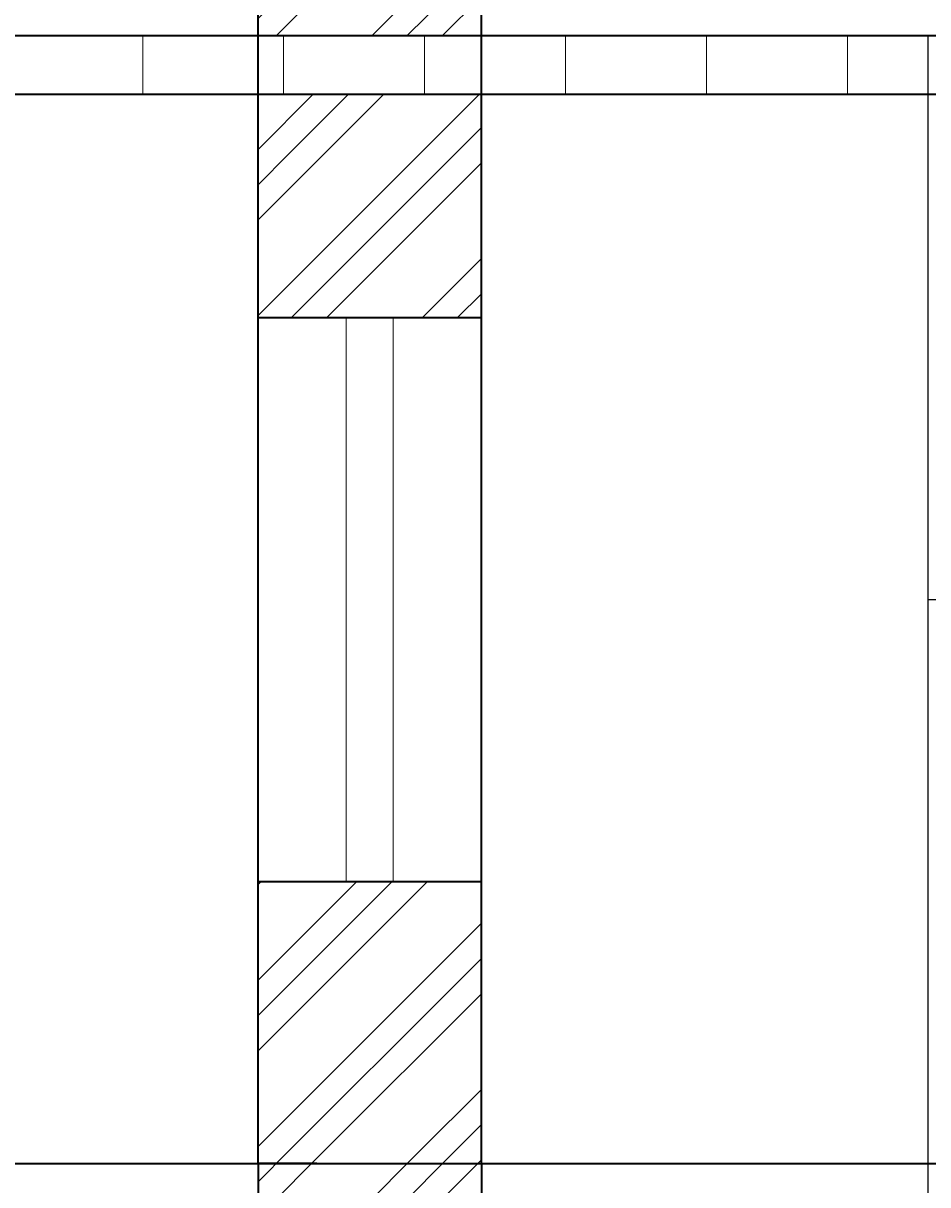
# Model space of a CAD drawing. Units: inches. Extents: x -128 to 854, y -395 to 398.
# Tile 14 of 61: x 122 to 199, y -300 to -201. Entities that reach past the tile are written whole.
import ezdxf

# ---------------------------------------------------------------- set-up
doc = ezdxf.new("R2010")
doc.units = ezdxf.units.IN
doc.header["$MEASUREMENT"] = 0
for name, color, linetype, lineweight in [('A-ANNO-DIMS', 2, 'Continuous', 18), ('A-GLAZ', 220, 'Continuous', 18), ('A-SECT', 220, 'Continuous', 35), ('A-SECT-PATT', 8, 'Continuous', 13), ('S-FNDN', 2, 'Continuous', 35)]:
    doc.layers.add(name, color=color, linetype=linetype, lineweight=lineweight)
doc.styles.get("Standard").update_dxf_attribs({"font": 'arial.ttf'})
doc.dimstyles.get("Standard").update_dxf_attribs({"dimtxt": 0.18, "dimasz": 0.18, "dimexe": 0.18, "dimexo": 0.0625, "dimgap": 0.09, "dimtad": 0, "dimtih": 1, "dimtoh": 1, "dimdec": 1, "dimzin": 0, "dimdsep": 46, "dimlunit": 4, "dimtxsty": 'Standard', "dimcen": 0.09, "dimclrd": 1, "dimclre": 2, "dimclrt": 6, "dimadec": 0, "dimazin": 0, "dimtfac": 1, "dimtdec": 1, "dimtofl": 0, "dimtmove": 0, "dimatfit": 3, "dimfxl": 1, "dimtfill": 2, "dimtfillclr": 3, "dimtolj": 1, "dimtzin": 0, "dimarcsym": 0})
pattern_1 = [(45, (0, 0), (14.14214, -9e-16), [20]), (45, (3, 0), (14.14214, -9e-16), [20]), (45, (6, 0), (14.14214, -9e-16), [20])]

# ---------------------------------------------------------------- blocks, each defined once
blk = doc.blocks.new('*D126')
at = {"layer": 'A-ANNO-DIMS', "color": 2, "lineweight": -2, "transparency": 16777216}
for p, q in [((160.839, -178.082), (160.839, -381.899)), ((198.839, -202.082), (198.839, -381.899))]:
    blk.add_line(p, q, dxfattribs=at)
at = {"layer": 'A-ANNO-DIMS', "color": 1, "lineweight": -2, "transparency": 16777216}
for p, q in [((161.019, -381.719), (179.51, -381.719)), ((198.659, -381.719), (180.168, -381.719))]:
    blk.add_line(p, q, dxfattribs=at)
at = {"layer": 'A-ANNO-DIMS', "color": 1, "transparency": 16777216}
for points in [[(161.019, -381.689), (161.019, -381.749), (160.839, -381.719)], [(198.659, -381.689), (198.659, -381.749), (198.839, -381.719)]]:
    blk.add_solid(points, dxfattribs=at)
at = {"layer": 'Defpoints', "color": 0, "transparency": 16777216}
for p in [(160.839, -178.019), (198.839, -202.019), (198.839, -381.719)]:
    blk.add_point(p, dxfattribs=at)
at = {"layer": 'A-ANNO-DIMS', "color": 6, "transparency": 16777216, "insert": (179.839, -381.719), "char_height": 0.18, "attachment_point": 5, "bg_fill": 1, "box_fill_scale": 1.25, "bg_fill_color": 3, "bg_fill_transparency": 0}
blk.add_mtext('\\A1;3\'-2"', dxfattribs=at)
blk = doc.blocks.new('*D132')
at = {"layer": 'A-ANNO-DIMS', "color": 2, "lineweight": -2, "transparency": 16777216}
for p, q in [((198.902, -250.019), (389.719, -250.019)), ((160.902, -298.019), (389.719, -298.019))]:
    blk.add_line(p, q, dxfattribs=at)
at = {"layer": 'A-ANNO-DIMS', "color": 1, "lineweight": -2, "transparency": 16777216}
for p, q in [((389.539, -250.199), (389.539, -273.837)), ((389.539, -297.839), (389.539, -274.201))]:
    blk.add_line(p, q, dxfattribs=at)
at = {"layer": 'A-ANNO-DIMS', "color": 1, "transparency": 16777216}
for points in [[(389.509, -250.199), (389.569, -250.199), (389.539, -250.019)], [(389.509, -297.839), (389.569, -297.839), (389.539, -298.019)]]:
    blk.add_solid(points, dxfattribs=at)
at = {"layer": 'Defpoints', "color": 0, "transparency": 16777216}
for p in [(198.839, -250.019), (389.539, -250.019), (160.839, -298.019)]:
    blk.add_point(p, dxfattribs=at)
at = {"layer": 'A-ANNO-DIMS', "color": 6, "transparency": 16777216, "insert": (389.539, -274.019), "char_height": 0.18, "attachment_point": 5, "bg_fill": 1, "box_fill_scale": 1.25, "bg_fill_color": 3, "bg_fill_transparency": 0}
blk.add_mtext('\\A1;4\'-0"', dxfattribs=at)

msp = doc.modelspace()

# ---------------------------------------------------------------- hatches: boundary and pattern name
at = {"layer": 'A-SECT-PATT'}
h = msp.add_hatch(dxfattribs=at)
h.set_pattern_fill('GOST_GROUND', color=256)
h.set_pattern_definition(pattern_1)
h.paths.add_polyline_path([(-37.161, -178.019), (-56.161, -178.019), (-56.161, -202.019), (-37.161, -202.019)])
h.paths.add_polyline_path([(160.839, -178.019), (141.839, -178.019), (141.839, -202.019), (160.839, -202.019)])
h.paths.add_polyline_path([(160.839, -207.019), (141.839, -207.019), (141.839, -226.019), (160.839, -226.019)])
h.paths.add_polyline_path([(317.839, -178.019), (298.839, -178.019), (298.839, -202.019), (317.839, -202.019)])
h.paths.add_polyline_path([(317.839, -207.019), (298.839, -207.019), (298.839, -226.019), (317.839, -226.019)])
h.paths.add_polyline_path([(317.839, -274.019), (298.839, -274.019), (298.839, -298.019), (303.839, -298.019), (312.839, -298.019), (317.839, -298.019)])
h = msp.add_hatch(dxfattribs=at)
h.set_pattern_fill('ANSI31', color=256, scale=96, angle=45, style=0)
h.paths.add_polyline_path([(-38.361, -202.019), (300.039, -202.019), (300.039, -207.019), (-38.361, -207.019)])
h = msp.add_hatch(dxfattribs=at)
h.set_pattern_fill('GOST_GROUND', color=256)
h.set_pattern_definition(pattern_1)
h.paths.add_polyline_path([(-27.161, -322.019), (-37.161, -322.019), (-37.161, -298.019), (-56.161, -298.019), (-56.161, -322.019), (-66.161, -322.019), (-66.161, -346.019), (-27.161, -346.019)])
h.paths.add_polyline_path([(170.839, -322.019), (160.839, -322.019), (160.839, -298.019), (155.839, -298.019), (141.839, -298.019), (141.839, -322.019), (131.839, -322.019), (131.839, -346.019), (170.839, -346.019)])
h.paths.add_polyline_path([(327.839, -322.019), (317.839, -322.019), (317.839, -298.019), (312.839, -298.019), (298.839, -298.019), (298.839, -322.019), (288.839, -322.019), (288.839, -346.019), (327.839, -346.019)])
h.paths.add_polyline_path([(-37.161, -274.019), (-56.161, -274.019), (-56.161, -298.019), (-37.161, -298.019)])
h.paths.add_polyline_path([(-37.161, -207.019), (-56.161, -207.019), (-56.161, -226.019), (-37.161, -226.019)])
h.paths.add_polyline_path([(160.839, -274.019), (141.839, -274.019), (141.839, -298.019), (155.839, -298.019), (160.839, -298.019)])

# ---------------------------------------------------------------- linework, layer by layer
at = {"layer": 'A-GLAZ'}
for p, q in [((149.339, -226.019), (149.339, -274.019)), ((153.339, -226.019), (153.339, -274.019))]:
    msp.add_line(p, q, dxfattribs=at)
at = {"layer": 'A-SECT'}
for p, q in [((141.839, -298.019), (141.839, -178.019)), ((160.839, -298.019), (160.839, -178.019)), ((-56.161, -202.019), (317.839, -202.019)), ((-56.161, -207.019), (317.839, -207.019)), ((141.839, -226.019), (160.839, -226.019)), ((141.839, -274.019), (160.839, -274.019)), ((-56.161, -298.019), (312.839, -298.019)), ((146.839, -298.019), (141.839, -298.019)), ((155.839, -298.019), (160.839, -298.019))]:
    msp.add_line(p, q, dxfattribs=at)
at = {"layer": 'S-FNDN'}
for p, q in [((146.839, -298.019), (141.839, -298.019)), ((141.839, -298.019), (141.839, -322.019)), ((155.839, -298.019), (160.839, -298.019)), ((160.839, -298.019), (160.839, -322.019))]:
    msp.add_line(p, q, dxfattribs=at)

# ---------------------------------------------------------------- dimensions: what is measured, and where the dimension line sits
at = {"layer": 'A-ANNO-DIMS'}
dim = msp.add_linear_dim(base=(198.839, -381.719), p1=(160.839, -178.019), p2=(198.839, -202.019), dimstyle='Standard', override={"dimdec": 1, "dimlfac": 1, "dimrnd": 0, "dimzin": 1, "dimdsep": 46, "dimlunit": 4, "dimfrac": 2}, dxfattribs=at)
dim.commit()
dim.dimension.update_dxf_attribs({"geometry": '*D126', "text_midpoint": (179.839, -381.719)})
dim = msp.add_linear_dim(base=(389.539, -250.019), p1=(160.839, -298.019), p2=(198.839, -250.019), angle=90, dimstyle='Standard', override={"dimdec": 1, "dimlfac": 1, "dimrnd": 0, "dimzin": 1, "dimdsep": 46, "dimlunit": 4, "dimfrac": 2}, dxfattribs=at)
dim.commit()
dim.dimension.update_dxf_attribs({"geometry": '*D132', "text_midpoint": (389.539, -274.019)})

doc.saveas('drawing.dxf')
